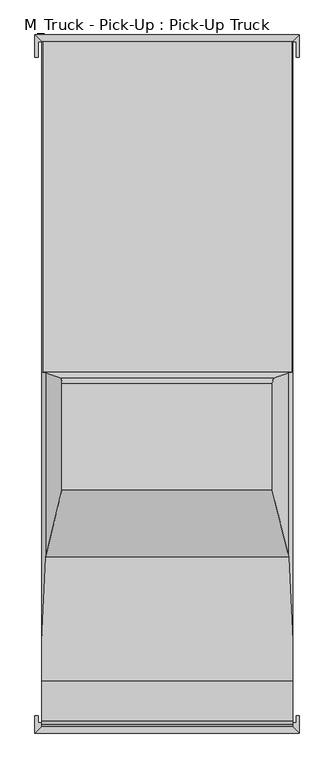
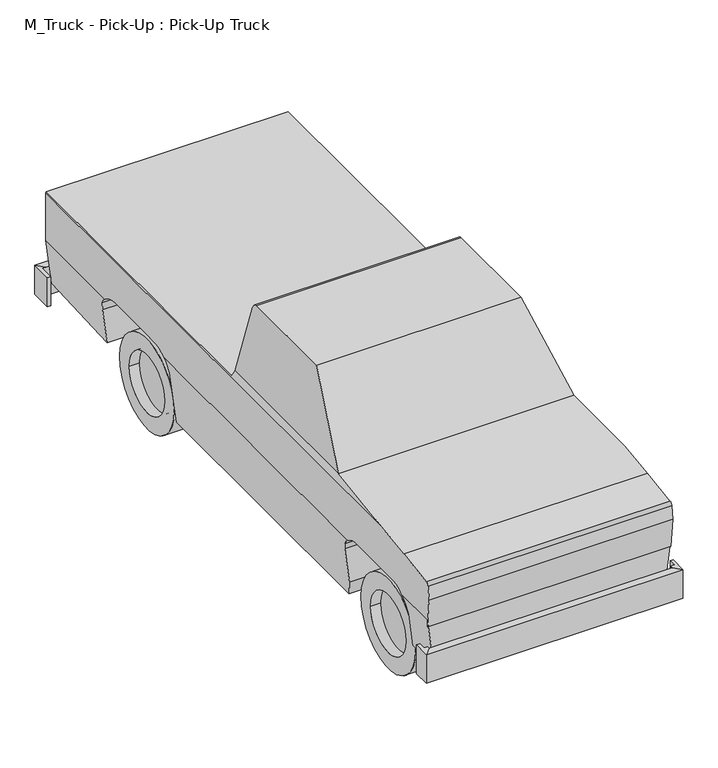
"""IFC4 building model written with IfcOpenShell, lengths in millimetres: geographic element geometry, M_Truck - Pick-Up : Pick-Up Truck."""

from ifc_helpers import new_model, si_unit, point, frame, frame_2d, origin, place, context, project, spatial, polyline, circle_curve, ellipse_curve, trimmed, segment, composite_curve, outline, extrude, faceted_brep, source, transform, mapped, element, save
from ifc_brep_helpers import plane_surface, cylinder_surface, revolved_surface, advanced_brep


def m_truck_pick_up_pick_up_truck_f485962c(model_context):
    return source(origin(), model_context, "Body", "SolidModel", [
        advanced_brep(
        [(-882.1615385, 2103.6156034, 888.7336798), (-882.1615385, 1697.2156034, 888.7336798), (-882.1615385, 1614.7015006, 885.1455636), (-882.1615385, 1473.5121228, 837.1131584), (-882.1615385, -912.9817492, 837.1131584), (-882.1615385, -1053.9517054, 878.8872426), (-882.1615385, -1474.8105853, 878.8872426), (-882.1615385, -1617.7834877, 837.1131584), (-882.1615385, -1951.924276, 837.1131584), (-882.1615385, -1951.924276, 779.2411665), (-882.1615385, -1975.8194827, 1006.5888718), (-882.1615385, -1963.4375574, 1107.4315608), (-882.1615385, -1939.9042038, 1130.9649145), (-882.1615385, -1644.5045632, 1173.526104), (-882.1615385, -1353.2454526, 1210.3079682), (-882.1615385, 3015.7615385, 1210.3079682), (-882.1615385, 3015.7615385, 837.1131584), (-882.1615385, 2243.9728923, 837.1131584), (946.6384615, -1644.5045632, 1173.526104), (946.6384615, -1939.9042038, 1130.9649145), (946.6384615, -1963.4375574, 1107.4315608), (946.6384615, -1975.8194827, 1006.5888718), (946.6384615, -1951.924276, 779.2411665), (946.6384615, -1951.924276, 837.1131584), (946.6384615, -1617.7834877, 837.1131584), (946.6384615, -1474.8105853, 878.8872426), (946.6384615, -1053.9517054, 878.8872426), (946.6384615, -912.9817492, 837.1131584), (946.6384615, 1473.5121228, 837.1131584), (946.6384615, 1614.7015006, 885.1455636), (946.6384615, 1697.2156034, 888.7336798), (946.6384615, 2103.6156034, 888.7336798), (946.6384615, 2243.9728923, 837.1131584), (946.6384615, 3015.7615385, 837.1131584), (946.6384615, 3015.7615385, 1210.3079682), (946.6384615, -1353.2454526, 1210.3079682), (-876.2843723, 3015.7615385, 1219.2), (940.7612953, 3015.7615385, 1219.2), (902.1686195, 3015.7615385, 480.544728), (-837.6916964, 3015.7615385, 480.544728), (897.0369558, 2300.369269, 439.3979826), (-832.5600327, 2300.369269, 439.3979826), (930.9047354, 2300.369269, 710.9568741), (-866.4278123, 2300.369269, 710.9568741), (939.4838124, 2288.2399438, 779.7456957), (-875.0068893, 2288.2399438, 779.7456957), (944.2646239, 1453.4521306, 818.079235), (-879.7877008, 1453.4521306, 818.079235), (935.7642918, 1419.378607, 749.921807), (-871.2873687, 1419.378607, 749.921807), (884.1769157, 1419.378607, 336.2835102), (-819.6999926, 1419.378607, 336.2835102), (884.1769157, -823.559725, 336.2835102), (-819.6999926, -823.559725, 336.2835102), (898.6478484, -854.6501227, 452.314454), (-834.1709253, -854.6501227, 452.314454), (933.4935408, -854.6501227, 731.714454), (-869.0166178, -854.6501227, 731.714454), (939.6132416, -867.7981302, 780.783486), (-875.1363185, -867.7981302, 780.783486), (930.9350571, -1682.962287, 711.2), (-866.458134, -1682.962287, 711.2), (899.0315641, -1682.962287, 455.3911665), (-834.554641, -1682.962287, 455.3911665), (899.0315641, -1951.924276, 455.3911665), (-834.554641, -1951.924276, 455.3911665), (939.4208895, -1951.924276, 779.2411665), (-874.9439664, -1951.924276, 779.2411665), (917.6799973, -743.8423581, 1254.1215299), (-853.2030742, -743.8423581, 1254.1215299), (800.2028589, -255.2503888, 1778.0), (-735.7259358, -255.2503888, 1778.0), (800.2028589, 522.1190782, 1778.0), (-735.7259358, 522.1190782, 1778.0), (-743.5250355, 560.0740962, 1743.2206338), (808.0019586, 560.0740962, 1743.2206338), (917.6799973, 602.8647232, 1254.1215299), (940.7612953, 605.9199612, 1219.2), (-876.2843723, 605.9199612, 1219.2), (-853.2030742, 602.8647232, 1254.1215299)],
        [
            (0, 1),
            (1, 2),
            (2, 3, circle_curve(frame((-882.1615385, 1606.9552598, 676.3888042), z_axis=(1.0, 0.0, 0.0), x_axis=(0.0, -1.0, 0.0)), 208.900428)),
            (3, 4),
            (4, 5, circle_curve(frame((-882.1615385, -1031.5575926, 695.7137663), z_axis=(1.0, 0.0, 0.0), x_axis=(0.0, -1.0, 0.0)), 184.5373098)),
            (5, 6),
            (6, 7, circle_curve(frame((-882.1615385, -1498.8876828, 695.7404401), z_axis=(1.0, 0.0, 0.0), x_axis=(0.0, -1.0, 0.0)), 184.7226513)),
            (7, 8),
            (8, 9),
            (9, 10),
            (10, 11),
            (11, 12, circle_curve(frame((-882.1615385, -1939.9042038, 1107.4315608), z_axis=(-1.0, 0.0, 0.0), x_axis=(0.0, -1.0, 0.0)), 23.5333537)),
            (12, 13),
            (13, 14, circle_curve(frame((-882.1615385, -446.5414344, -7141.0412638), z_axis=(-1.0, 0.0, 0.0), x_axis=(0.0, -1.0, 0.0)), 8400.4253566)),
            (14, 15),
            (15, 16),
            (16, 17),
            (17, 0, circle_curve(frame((-882.1615385, 2109.2327636, 687.3793785), z_axis=(1.0, 0.0, 0.0), x_axis=(0.0, -1.0, 0.0)), 201.4326367)),
            (18, 19),
            (19, 20, circle_curve(frame((946.6384615, -1939.9042038, 1107.4315608), z_axis=(1.0, 0.0, 0.0), x_axis=(0.0, -1.0, 0.0)), 23.5333537)),
            (20, 21),
            (21, 22),
            (22, 23),
            (23, 24),
            (24, 25, circle_curve(frame((946.6384615, -1498.8876828, 695.7404401), z_axis=(-1.0, 0.0, 0.0), x_axis=(0.0, -1.0, 0.0)), 184.7226513)),
            (25, 26),
            (26, 27, circle_curve(frame((946.6384615, -1031.5575926, 695.7137663), z_axis=(-1.0, 0.0, 0.0), x_axis=(0.0, -1.0, 0.0)), 184.5373098)),
            (27, 28),
            (28, 29, circle_curve(frame((946.6384615, 1606.9552598, 676.3888042), z_axis=(-1.0, 0.0, 0.0), x_axis=(0.0, -1.0, 0.0)), 208.900428)),
            (29, 30),
            (30, 31),
            (31, 32, circle_curve(frame((946.6384615, 2109.2327636, 687.3793785), z_axis=(-1.0, 0.0, 0.0), x_axis=(0.0, -1.0, 0.0)), 201.4326367)),
            (32, 33),
            (33, 34),
            (34, 35),
            (35, 18, circle_curve(frame((946.6384615, -446.5414344, -7141.0412638), z_axis=(1.0, 0.0, 0.0), x_axis=(0.0, -1.0, 0.0)), 8400.4253566)),
            (15, 36),
            (36, 37),
            (37, 34),
            (33, 38),
            (38, 39),
            (39, 16),
            (38, 40),
            (40, 41),
            (41, 39),
            (40, 42),
            (42, 43),
            (43, 41),
            (42, 44),
            (44, 45),
            (45, 43),
            (31, 0),
            (17, 45, ellipse_curve(frame((-863.4873178, 2109.2327636, 687.3793785), z_axis=(-0.9923125046981085, 0.0, -0.12375739581845786), x_axis=(0.12375739581845774, 0.0, -0.9923125046981085)), 202.9931455, 201.4326367)),
            (44, 32, ellipse_curve(frame((927.9642409, 2109.2327636, 687.3793785), z_axis=(0.992312504698106, 0.0, -0.12375739581847864), x_axis=(0.12375739581847735, 0.0, 0.9923125046981061)), 202.9931455, 201.4326367)),
            (30, 1),
            (29, 2),
            (28, 46, ellipse_curve(frame((926.5935388, 1606.9552598, 676.3888042), z_axis=(0.992312504698106, 0.0, -0.12375739581847864), x_axis=(0.12375739581847735, 0.0, 0.9923125046981061)), 210.5187902, 208.900428)),
            (46, 47),
            (47, 3, ellipse_curve(frame((-862.1166157, 1606.9552598, 676.3888042), z_axis=(-0.9923125046981085, 0.0, -0.12375739581845786), x_axis=(0.12375739581845774, 0.0, -0.9923125046981085)), 210.5187902, 208.900428)),
            (46, 48),
            (48, 49),
            (49, 47),
            (48, 50),
            (50, 51),
            (51, 49),
            (50, 52),
            (52, 53),
            (53, 51),
            (52, 54),
            (54, 55),
            (55, 53),
            (54, 56),
            (56, 57),
            (57, 55),
            (56, 58),
            (58, 59),
            (59, 57),
            (26, 5),
            (4, 59, ellipse_curve(frame((-864.5267506, -1031.5575926, 695.7137663), z_axis=(-0.9923125046981085, 0.0, -0.12375739581845786), x_axis=(0.12375739581845774, 0.0, -0.9923125046981085)), 185.9669297, 184.5373098)),
            (58, 27, ellipse_curve(frame((929.0036737, -1031.5575926, 695.7137663), z_axis=(0.992312504698106, 0.0, -0.12375739581847864), x_axis=(0.12375739581847735, 0.0, 0.9923125046981061)), 185.9669297, 184.5373098)),
            (25, 6),
            (24, 60, ellipse_curve(frame((929.0070003, -1498.8876828, 695.7404401), z_axis=(0.992312504698106, 0.0, -0.12375739581847864), x_axis=(0.12375739581847735, 0.0, 0.9923125046981061)), 186.153707, 184.7226513)),
            (60, 61),
            (61, 7, ellipse_curve(frame((-864.5300772, -1498.8876828, 695.7404401), z_axis=(-0.9923125046981085, 0.0, -0.12375739581845786), x_axis=(0.12375739581845774, 0.0, -0.9923125046981085)), 186.153707, 184.7226513)),
            (60, 62),
            (62, 63),
            (63, 61),
            (62, 64),
            (64, 65),
            (65, 63),
            (64, 66),
            (66, 67),
            (67, 65),
            (9, 67),
            (66, 22),
            (21, 10),
            (20, 11),
            (19, 12),
            (18, 13),
            (35, 68, ellipse_curve(frame((6466.4418903, -446.5414344, -7141.0412638), z_axis=(-0.8342458244432318, 0.0, -0.5513926952717387), x_axis=(-0.5513926952717385, 0.0, 0.8342458244432318)), 10069.4844499, 8400.4253566)),
            (68, 69),
            (69, 14, ellipse_curve(frame((-6401.9649673, -446.5414344, -7141.0412638), z_axis=(0.8342458244429898, 0.0, -0.5513926952721048), x_axis=(-0.5513926952721048, 0.0, -0.8342458244429898)), 10069.4844499, 8400.4253566)),
            (68, 70),
            (70, 71),
            (71, 69),
            (70, 72),
            (72, 73),
            (73, 71),
            (74, 75),
            (75, 76),
            (76, 77),
            (77, 78),
            (78, 79),
            (79, 74),
            (36, 78),
            (77, 37),
            (8, 67),
            (66, 23),
            (69, 79),
            (73, 74, ellipse_curve(frame((-744.2696711, 522.1190782, 1739.9), z_axis=(-0.9757672710776872, 0.0, 0.21881095195077252), x_axis=(-0.21881095195077238, 0.0, -0.9757672710776871)), 39.0461959, 38.1)),
            (68, 76),
            (75, 72, ellipse_curve(frame((808.7465942, 522.1190782, 1739.9), z_axis=(0.9757672710776958, 0.0, 0.21881095195073466), x_axis=(-0.21881095195073416, 0.0, 0.9757672710776959)), 39.0461959, 38.1)),
        ],
        [
            plane_surface(frame((-882.1615385, 3015.7615385, 480.544728), z_axis=(-1.0, 0.0, 0.0), x_axis=(0.0, 0.0, -1.0))),
            plane_surface(frame((946.6384615, 3015.7615385, 480.544728), z_axis=(1.0, 0.0, 0.0), x_axis=(0.0, 0.0, 1.0))),
            plane_surface(frame((-882.1615385, 3015.7615385, 1219.2), z_axis=(0.0, 1.0, 0.0), x_axis=(1.0, 0.0, 0.0))),
            plane_surface(frame((-882.1615385, 3015.7615385, 480.544728), z_axis=(0.0, 0.05742144008010288, -0.9983500279056075), x_axis=(1.0, 0.0, 0.0))),
            plane_surface(frame((-882.1615385, 2300.369269, 439.3979826), z_axis=(0.0, -1.0, 0.0), x_axis=(1.0, 0.0, 0.0))),
            plane_surface(frame((-882.1615385, 2300.369269, 710.9568741), z_axis=(0.0, -0.9848077530122078, -0.17364817766693216), x_axis=(1.0, 0.0, 0.0))),
            revolved_surface(polyline([(953.0861439560813, 1907.8001269000001, 687.3793785), (-888.6092208560774, 1907.8001269000001, 687.3793785)]), (946.6384615, 2109.2327636, 687.3793785), (1.0, 0.0, 0.0)),
            plane_surface(frame((-882.1615385, 2103.6156034, 888.7336798), z_axis=(0.0, 0.0, -1.0), x_axis=(1.0, 0.0, 0.0))),
            plane_surface(frame((-882.1615385, 1697.2156034, 888.7336798), z_axis=(0.0, 0.04344382849430752, -0.9990558711932768), x_axis=(1.0, 0.0, 0.0))),
            revolved_surface(polyline([(952.6467960460084, 1398.0548318, 676.3888042), (-888.1698729460043, 1398.0548318, 676.3888042)]), (946.6384615, 1606.9552598, 676.3888042), (1.0, 0.0, 0.0)),
            plane_surface(frame((-882.1615385, 1453.4521306, 818.079235), z_axis=(0.0, 0.8944544352885822, -0.44715910277280924), x_axis=(1.0, 0.0, 0.0))),
            plane_surface(frame((-882.1615385, 1419.378607, 749.921807), z_axis=(0.0, 1.0, 0.0), x_axis=(1.0, 0.0, 0.0))),
            plane_surface(frame((-882.1615385, 1419.378607, 336.2835102), z_axis=(0.0, 0.0, -1.0), x_axis=(1.0, 0.0, 0.0))),
            plane_surface(frame((-882.1615385, -823.559725, 336.2835102), z_axis=(0.0, -0.965925826289069, -0.2588190451025183), x_axis=(1.0, 0.0, 0.0))),
            plane_surface(frame((-882.1615385, -854.6501227, 452.314454), z_axis=(0.0, -1.0, 0.0), x_axis=(1.0, 0.0, 0.0))),
            plane_surface(frame((-882.1615385, -854.6501227, 731.714454), z_axis=(0.0, -0.9659258262890823, -0.25881904510246856), x_axis=(1.0, 0.0, 0.0))),
            revolved_surface(polyline([(952.0184566280299, -1216.0949024, 695.7137663), (-887.5415335280263, -1216.0949024, 695.7137663)]), (946.6384615, -1031.5575926, 695.7137663), (1.0, 0.0, 0.0)),
            plane_surface(frame((-882.1615385, -1053.9517054, 878.8872426), z_axis=(0.0, 0.0, -1.0), x_axis=(1.0, 0.0, 0.0))),
            revolved_surface(polyline([(952.0448983002758, -1683.6103341, 695.7404401), (-887.5679752002723, -1683.6103341, 695.7404401)]), (946.6384615, -1498.8876828, 695.7404401), (1.0, 0.0, 0.0)),
            plane_surface(frame((-882.1615385, -1682.962287, 711.2), z_axis=(0.0, 1.0, 0.0), x_axis=(1.0, 0.0, 0.0))),
            plane_surface(frame((-882.1615385, -1682.962287, 455.3911665), z_axis=(0.0, 0.0, -1.0), x_axis=(1.0, 0.0, 0.0))),
            plane_surface(frame((-882.1615385, -1951.924276, 455.3911665), z_axis=(0.0, -1.0, 0.0), x_axis=(1.0, 0.0, 0.0))),
            plane_surface(frame((-882.1615385, -1951.924276, 779.2411665), z_axis=(0.0, -0.9945218953682735, -0.10452846326765221), x_axis=(1.0, 0.0, 0.0))),
            plane_surface(frame((-882.1615385, -1975.8194827, 1006.5888718), z_axis=(0.0, -0.9925461516413229, 0.1218693434051412), x_axis=(1.0, 0.0, 0.0))),
            cylinder_surface(frame((946.6384615, -1939.9042038, 1107.4315608), z_axis=(-1.0, 0.0, 0.0), x_axis=(0.0, -1.0, 0.0)), 23.5333537),
            plane_surface(frame((-882.1615385, -1939.9042038, 1130.9649145), z_axis=(0.0, -0.1426074368747531, 0.9897793284101327), x_axis=(1.0, 0.0, 0.0))),
            cylinder_surface(frame((946.6384615, -446.5414344, -7141.0412638), z_axis=(-1.0, 0.0, 0.0), x_axis=(0.0, -1.0, 0.0)), 8400.4253566),
            plane_surface(frame((-882.1615385, -743.8423581, 1254.1215299), z_axis=(0.0, -0.7313067761874522, 0.6820486779565779), x_axis=(1.0, 0.0, 0.0))),
            plane_surface(frame((-882.1615385, -255.2503888, 1778.0), z_axis=(0.0, 0.0, 1.0), x_axis=(1.0, 0.0, 0.0))),
            plane_surface(frame((-882.1615385, 560.0740962, 1743.2206338), z_axis=(0.0, 0.9961946980917455, 0.08715574274765842), x_axis=(1.0, 0.0, 0.0))),
            plane_surface(frame((-882.1615385, 605.9199612, 1219.2), z_axis=(0.0, 0.0, 1.0), x_axis=(1.0, 0.0, 0.0))),
            plane_surface(frame((-730.4934031, -1951.924276, 305.3311322), z_axis=(0.0, 1.0, 0.0), x_axis=(1.0, 0.0, 0.0))),
            plane_surface(frame((-815.8397312, -1951.924276, 305.3311322), z_axis=(-0.9923125046981085, 0.0, -0.12375739581845786), x_axis=(0.0, 1.0, 0.0))),
            plane_surface(frame((-884.2900076, -1951.924276, 1207.0876381), z_axis=(-0.8342458244429898, 0.0, 0.5513926952721048), x_axis=(0.0, 1.0, 0.0))),
            plane_surface(frame((-853.2030742, -1951.924276, 1254.1215299), z_axis=(-0.9757672710776872, 0.0, 0.21881095195077252), x_axis=(0.0, 1.0, 0.0))),
            plane_surface(frame((800.2028589, -1951.924276, 1778.0), z_axis=(0.9757672710776958, 0.0, 0.21881095195073466), x_axis=(0.0, 1.0, 0.0))),
            plane_surface(frame((917.6799973, -1951.924276, 1254.1215299), z_axis=(0.8342458244432318, 0.0, 0.5513926952717387), x_axis=(0.0, 1.0, 0.0))),
            plane_surface(frame((948.7669307, -1951.924276, 854.1796662), z_axis=(0.992312504698106, 0.0, -0.12375739581847864), x_axis=(0.0, 1.0, 0.0))),
            cylinder_surface(frame((946.6384615, 522.1190782, 1739.9), z_axis=(-1.0, 0.0, 0.0), x_axis=(0.0, -1.0, 0.0)), 38.1),
        ],
        [
            (0, [[1, 2, 3, 4, 5, 6, 7, 8, 9, 10, 11, 12, 13, 14, 15, 16, 17, 18]]),
            (1, [[19, 20, 21, 22, 23, 24, 25, 26, 27, 28, 29, 30, 31, 32, 33, 34, 35, 36]]),
            (2, [[-16, 37, 38, 39, -34, 40, 41, 42]]),
            (3, [[-41, 43, 44, 45]]),
            (4, [[-44, 46, 47, 48]]),
            (5, [[-47, 49, 50, 51]]),
            (6, [[52, -18, 53, -50, 54, -32]]),
            (7, [[-1, -52, -31, 55]]),
            (8, [[-2, -55, -30, 56]]),
            (9, [[-56, -29, 57, 58, 59, -3]]),
            (10, [[-58, 60, 61, 62]]),
            (11, [[-61, 63, 64, 65]]),
            (12, [[-64, 66, 67, 68]]),
            (13, [[-67, 69, 70, 71]]),
            (14, [[-70, 72, 73, 74]]),
            (15, [[-73, 75, 76, 77]]),
            (16, [[78, -5, 79, -76, 80, -27]]),
            (17, [[-6, -78, -26, 81]]),
            (18, [[-81, -25, 82, 83, 84, -7]]),
            (19, [[-83, 85, 86, 87]]),
            (20, [[-86, 88, 89, 90]]),
            (21, [[-89, 91, 92, 93]]),
            (22, [[-10, 94, -92, 95, -22, 96]]),
            (23, [[-11, -96, -21, 97]]),
            (24, [[-12, -97, -20, 98]]),
            (25, [[-13, -98, -19, 99]]),
            (26, [[-99, -36, 100, 101, 102, -14]]),
            (27, [[-101, 103, 104, 105]]),
            (28, [[-104, 106, 107, 108]]),
            (29, [[109, 110, 111, 112, 113, 114]]),
            (30, [[-38, 115, -112, 116]]),
            (31, [[117, -94, -9]]),
            (31, [[118, -23, -95]]),
            (32, [[-4, -59, -62, -65, -68, -71, -74, -77, -79]]),
            (32, [[-17, -42, -45, -48, -51, -53]]),
            (32, [[-117, -8, -84, -87, -90, -93]]),
            (33, [[119, -113, -115, -37, -15, -102]]),
            (34, [[-119, -105, -108, 120, -114]]),
            (35, [[121, -110, 122, -106, -103]]),
            (36, [[-121, -100, -35, -39, -116, -111]]),
            (37, [[-28, -80, -75, -72, -69, -66, -63, -60, -57]]),
            (37, [[-33, -54, -49, -46, -43, -40]]),
            (37, [[-118, -91, -88, -85, -82, -24]]),
            (38, [[-107, -122, -109, -120]]),
        ],
    ),
        faceted_brep([(-932.9615385, -1899.6194827, 394.7577003), (-932.9615385, -1899.6194827, 623.3577003), (-907.5615385, -1899.6194827, 623.3577003), (-907.5615385, -1899.6194827, 394.7577003), (-932.9615385, -2026.6194827, 394.7577003), (-932.9615385, -2026.6194827, 623.3577003), (-882.1615385, -1975.8194827, 623.3577003), (-882.1615385, -1951.924276, 623.3577003), (-907.5615385, -1951.924276, 623.3577003), (-882.1615385, -1975.8194827, 394.7577003), (-882.1615385, -1951.924276, 394.7577003), (-907.5615385, -1951.924276, 394.7577003), (993.9251801, -2026.6194827, 394.7577003), (993.9251801, -2026.6194827, 623.3577003), (943.1251801, -1975.8194827, 623.3577003), (943.1251801, -1975.8194827, 394.7577003), (993.9251801, -1899.6194827, 623.3577003), (993.9251801, -1899.6194827, 394.7577003), (972.0384615, -1899.6194827, 394.7577003), (972.0384615, -1899.6194827, 623.3577003), (972.0384615, -1951.924276, 623.3577003), (943.1251801, -1951.924276, 623.3577003), (943.1251801, -1951.924276, 394.7577003), (972.0384615, -1951.924276, 394.7577003)], [[[0, 1, 2, 3]], [[1, 0, 4, 5]], [[1, 5, 6, 7, 8, 2]], [[6, 9, 10, 7]], [[4, 0, 3, 11, 10, 9]], [[5, 4, 12, 13]], [[6, 5, 13, 14]], [[9, 6, 14, 15]], [[4, 9, 15, 12]], [[16, 17, 18, 19]], [[13, 12, 17, 16]], [[14, 13, 16, 19, 20, 21]], [[15, 14, 21, 22]], [[12, 15, 22, 23, 18, 17]], [[11, 8, 7, 10]], [[20, 23, 22, 21]], [[8, 11, 3, 2]], [[23, 20, 19, 18]]]),
        faceted_brep([(-932.9615385, 2903.0203063, 623.3577003), (-932.9615385, 2903.0203063, 394.7577003), (-907.5615385, 2903.0203063, 394.7577003), (-907.5615385, 2903.0203063, 623.3577003), (-932.9615385, 3066.5615385, 394.7577003), (-882.1615385, 3015.7615385, 394.7577003), (-907.5615385, 3015.7615385, 394.7577003), (-882.1615385, 3015.7615385, 623.3577003), (-932.9615385, 3066.5615385, 623.3577003), (-907.5615385, 3015.7615385, 623.3577003), (943.1251801, 3015.7615385, 394.7577003), (993.9251801, 3066.5615385, 394.7577003), (972.0384615, 3015.7615385, 394.7577003), (972.0384615, 3015.7615385, 623.3577003), (943.1251801, 3015.7615385, 623.3577003), (993.9251801, 3066.5615385, 623.3577003), (993.9251801, 2903.0203063, 394.7577003), (993.9251801, 2903.0203063, 623.3577003), (972.0384615, 2903.0203063, 623.3577003), (972.0384615, 2903.0203063, 394.7577003)], [[[0, 1, 2, 3]], [[1, 4, 5, 6, 2]], [[7, 8, 0, 3, 9]], [[1, 0, 8, 4]], [[10, 5, 4, 11]], [[10, 12, 13, 14, 7, 9, 6, 5]], [[8, 7, 14, 15]], [[4, 8, 15, 11]], [[16, 17, 18, 19]], [[10, 11, 16, 19, 12]], [[15, 14, 13, 18, 17]], [[11, 15, 17, 16]], [[6, 9, 3, 2]], [[13, 12, 19, 18]]]),
        extrude(outline(composite_curve([segment(trimmed(circle_curve(frame_2d((1872.7733891, 355.6)), 355.6), [point((1517.1733891, 355.6))], [point((2228.3733891, 355.6))], False, "CARTESIAN"), True, "CONTINUOUS"), segment(trimmed(circle_curve(frame_2d((1872.7733891, 355.6)), 355.6), [point((2228.3733891, 355.6))], [point((1517.1733891, 355.6))], False, "CARTESIAN"), True, "CONTINUOUS")], self_intersect=False), holes=[composite_curve([segment(trimmed(circle_curve(frame_2d((1872.7733891, 355.6)), 228.6), [point((2101.3733891, 355.6))], [point((1644.1733891, 355.6))], True, "CARTESIAN"), True, "CONTINUOUS"), segment(trimmed(circle_curve(frame_2d((1872.7733891, 355.6)), 228.6), [point((1644.1733891, 355.6))], [point((2101.3733891, 355.6))], True, "CARTESIAN"), True, "CONTINUOUS")], self_intersect=False)]), frame((-780.5615385, 0.0, 0.0), z_axis=(1.0, 0.0, 0.0), x_axis=(0.0, 1.0, 0.0)), (0.0, 0.0, 1.0), 203.2),
        extrude(outline(composite_curve([segment(trimmed(circle_curve(frame_2d((-1267.5375629, 355.6)), 355.6), [point((-911.9375629, 355.6))], [point((-1623.1375629, 355.6))], False, "CARTESIAN"), True, "CONTINUOUS"), segment(trimmed(circle_curve(frame_2d((-1267.5375629, 355.6)), 355.6), [point((-1623.1375629, 355.6))], [point((-911.9375629, 355.6))], False, "CARTESIAN"), True, "CONTINUOUS")], self_intersect=False), holes=[composite_curve([segment(trimmed(circle_curve(frame_2d((-1267.5375629, 355.6)), 228.6), [point((-1038.9375629, 355.6))], [point((-1496.1375629, 355.6))], True, "CARTESIAN"), True, "CONTINUOUS"), segment(trimmed(circle_curve(frame_2d((-1267.5375629, 355.6)), 228.6), [point((-1496.1375629, 355.6))], [point((-1038.9375629, 355.6))], True, "CARTESIAN"), True, "CONTINUOUS")], self_intersect=False)]), frame((-780.5615385, 0.0, 0.0), z_axis=(1.0, 0.0, 0.0), x_axis=(0.0, 1.0, 0.0)), (0.0, 0.0, 1.0), 203.2),
        extrude(outline(polyline([(520.2761241, 2300.369269), (520.2761241, 1419.378607), (-437.7696481, 1419.378607), (-437.7696481, 2300.369269), (520.2761241, 2300.369269)])), frame((0.0, 0.0, 595.9078125), z_axis=(0.0, 0.0, 1.0), x_axis=(1.0, 0.0, 0.0)), (0.0, 0.0, 1.0), 27.7189478),
        extrude(outline(composite_curve([segment(polyline([(2300.369269, 456.9336798), (1419.378607, 456.9336798), (1419.378607, 749.921807), (1453.4521306, 818.079235)]), True, "CONTINUOUS"), segment(trimmed(circle_curve(frame_2d((1606.9552598, 676.3888042)), 208.900428), [point((1453.4521306, 818.079235))], [point((1614.7015006, 885.1455636))], False, "CARTESIAN"), True, "CONTINUOUS"), segment(polyline([(1614.7015006, 885.1455636), (1697.2156034, 888.7336798), (2103.6156034, 888.7336798)]), True, "CONTINUOUS"), segment(trimmed(circle_curve(frame_2d((2109.2327636, 687.3793785)), 201.4326367), [point((2103.6156034, 888.7336798))], [point((2288.2399438, 779.7456957))], False, "CARTESIAN"), True, "CONTINUOUS"), segment(polyline([(2288.2399438, 779.7456957), (2300.369269, 710.9568741), (2300.369269, 456.9336798)]), True, "CONTINUOUS")], self_intersect=False)), frame((-484.8485994, 0.0, 0.0), z_axis=(1.0, 0.0, 0.0), x_axis=(0.0, 1.0, 0.0)), (0.0, 0.0, 1.0), 47.0684735),
        extrude(outline(composite_curve([segment(polyline([(2300.369269, 456.9336798), (1419.378607, 456.9336798), (1419.378607, 749.921807), (1453.4521306, 818.079235)]), True, "CONTINUOUS"), segment(trimmed(circle_curve(frame_2d((1606.9552598, 676.3888042)), 208.900428), [point((1453.4521306, 818.079235))], [point((1614.7015006, 885.1455636))], False, "CARTESIAN"), True, "CONTINUOUS"), segment(polyline([(1614.7015006, 885.1455636), (1697.2156034, 888.7336798), (2103.6156034, 888.7336798)]), True, "CONTINUOUS"), segment(trimmed(circle_curve(frame_2d((2109.2327636, 687.3793785)), 201.4326367), [point((2103.6156034, 888.7336798))], [point((2288.2399438, 779.7456957))], False, "CARTESIAN"), True, "CONTINUOUS"), segment(polyline([(2288.2399438, 779.7456957), (2300.369269, 710.9568741), (2300.369269, 456.9336798)]), True, "CONTINUOUS")], self_intersect=False)), frame((520.2761241, 0.0, 0.0), z_axis=(1.0, 0.0, 0.0), x_axis=(0.0, 1.0, 0.0)), (0.0, 0.0, 1.0), 35.321875),
        extrude(outline(composite_curve([segment(trimmed(circle_curve(frame_2d((1872.7733891, 355.6)), 228.6), [point((1644.1733891, 355.6))], [point((2101.3733891, 355.6))], False, "CARTESIAN"), True, "CONTINUOUS"), segment(trimmed(circle_curve(frame_2d((1872.7733891, 355.6)), 228.6), [point((2101.3733891, 355.6))], [point((1644.1733891, 355.6))], False, "CARTESIAN"), True, "CONTINUOUS")], self_intersect=False)), frame((-705.0934031, 0.0, 0.0), z_axis=(1.0, 0.0, 0.0), x_axis=(0.0, 1.0, 0.0)), (0.0, 0.0, 1.0), 127.8117146),
        extrude(outline(composite_curve([segment(trimmed(circle_curve(frame_2d((-1267.5375629, 355.6)), 228.6), [point((-1496.1375629, 355.6))], [point((-1038.9375629, 355.6))], False, "CARTESIAN"), True, "CONTINUOUS"), segment(trimmed(circle_curve(frame_2d((-1267.5375629, 355.6)), 228.6), [point((-1038.9375629, 355.6))], [point((-1496.1375629, 355.6))], False, "CARTESIAN"), True, "CONTINUOUS")], self_intersect=False)), frame((-705.0934031, 0.0, 0.0), z_axis=(1.0, 0.0, 0.0), x_axis=(0.0, 1.0, 0.0)), (0.0, 0.0, 1.0), 127.8117146),
        extrude(outline(composite_curve([segment(trimmed(circle_curve(frame_2d((1872.7733891, 355.6)), 355.6), [point((1517.1733891, 355.6))], [point((2228.3733891, 355.6))], False, "CARTESIAN"), True, "CONTINUOUS"), segment(trimmed(circle_curve(frame_2d((1872.7733891, 355.6)), 355.6), [point((2228.3733891, 355.6))], [point((1517.1733891, 355.6))], False, "CARTESIAN"), True, "CONTINUOUS")], self_intersect=False), holes=[composite_curve([segment(trimmed(circle_curve(frame_2d((1872.7733891, 355.6)), 228.6), [point((2101.3733891, 355.6))], [point((1644.1733891, 355.6))], True, "CARTESIAN"), True, "CONTINUOUS"), segment(trimmed(circle_curve(frame_2d((1872.7733891, 355.6)), 228.6), [point((1644.1733891, 355.6))], [point((2101.3733891, 355.6))], True, "CARTESIAN"), True, "CONTINUOUS")], self_intersect=False)]), frame((641.8384615, 0.0, 0.0), z_axis=(1.0, 0.0, 0.0), x_axis=(0.0, 1.0, 0.0)), (0.0, 0.0, 1.0), 203.2),
        extrude(outline(composite_curve([segment(trimmed(circle_curve(frame_2d((-1267.5375629, 355.6)), 355.6), [point((-911.9375629, 355.6))], [point((-1623.1375629, 355.6))], False, "CARTESIAN"), True, "CONTINUOUS"), segment(trimmed(circle_curve(frame_2d((-1267.5375629, 355.6)), 355.6), [point((-1623.1375629, 355.6))], [point((-911.9375629, 355.6))], False, "CARTESIAN"), True, "CONTINUOUS")], self_intersect=False), holes=[composite_curve([segment(trimmed(circle_curve(frame_2d((-1267.5375629, 355.6)), 228.6), [point((-1038.9375629, 355.6))], [point((-1496.1375629, 355.6))], True, "CARTESIAN"), True, "CONTINUOUS"), segment(trimmed(circle_curve(frame_2d((-1267.5375629, 355.6)), 228.6), [point((-1496.1375629, 355.6))], [point((-1038.9375629, 355.6))], True, "CARTESIAN"), True, "CONTINUOUS")], self_intersect=False)]), frame((641.8384615, 0.0, 0.0), z_axis=(1.0, 0.0, 0.0), x_axis=(0.0, 1.0, 0.0)), (0.0, 0.0, 1.0), 203.2),
        extrude(outline(composite_curve([segment(trimmed(circle_curve(frame_2d((1872.7733891, 355.6)), 228.6), [point((1644.1733891, 355.6))], [point((2101.3733891, 355.6))], False, "CARTESIAN"), True, "CONTINUOUS"), segment(trimmed(circle_curve(frame_2d((1872.7733891, 355.6)), 228.6), [point((2101.3733891, 355.6))], [point((1644.1733891, 355.6))], False, "CARTESIAN"), True, "CONTINUOUS")], self_intersect=False)), frame((641.7586115, 0.0, 0.0), z_axis=(1.0, 0.0, 0.0), x_axis=(0.0, 1.0, 0.0)), (0.0, 0.0, 1.0), 127.8117146),
        extrude(outline(composite_curve([segment(trimmed(circle_curve(frame_2d((-1267.5375629, 355.6)), 228.6), [point((-1496.1375629, 355.6))], [point((-1038.9375629, 355.6))], False, "CARTESIAN"), True, "CONTINUOUS"), segment(trimmed(circle_curve(frame_2d((-1267.5375629, 355.6)), 228.6), [point((-1038.9375629, 355.6))], [point((-1496.1375629, 355.6))], False, "CARTESIAN"), True, "CONTINUOUS")], self_intersect=False)), frame((641.7586115, 0.0, 0.0), z_axis=(1.0, 0.0, 0.0), x_axis=(0.0, 1.0, 0.0)), (0.0, 0.0, 1.0), 127.8117146),
    ])


if __name__ == "__main__":
    model = new_model("IFC4")
    model_context = context("Model", 3, world=origin())
    ifc_project = project(units=[si_unit("LENGTHUNIT", "METRE", prefix="MILLI")], contexts=[model_context])
    site = spatial("IfcSite", under=ifc_project)
    building = spatial("IfcBuilding", under=site)
    placement = place(None, origin())
    m_truck_pick_up_pick_up_truck_shape = m_truck_pick_up_pick_up_truck_f485962c(model_context)
    element("IfcGeographicElement", 1, ObjectType="M_Truck - Pick-Up : Pick-Up Truck", at=placement, inside=building, context=model_context, shape_type="MappedRepresentation", body=[
        mapped(m_truck_pick_up_pick_up_truck_shape, transform((0.0, 0.0, 0.0), x_axis=(1.0, 0.0, 0.0), y_axis=(0.0, 1.0, 0.0), z_axis=(0.0, 0.0, 1.0))),
    ])
    save(model, "model.ifc")

# Revit data of these elements
# Type "M_Truck - Pick-Up : Pick-Up Truck"
#   Tire Material = Rubber - Black
#   Material = Metal - Paint Finish - Blue, Sky
# Element 1 (IfcGeographicElement, "M_Truck - Pick-Up : Pick-Up Truck")
#   Materials on its faces: "Metal - Paint Finish - Blue, Sky", "Steel", "Rubber - Black"
# Materials
#   "Rubber - Black": class "Rubber", colour RGB 0 0 0, transparency 0
#   "Metal - Paint Finish - Blue, Sky": class "Paint", colour RGB 69 113 122, transparency 0
#   "Steel": class "Metal", colour RGB 128 128 128, transparency 0, Description = "Steel, mill finish", Cost = 0
